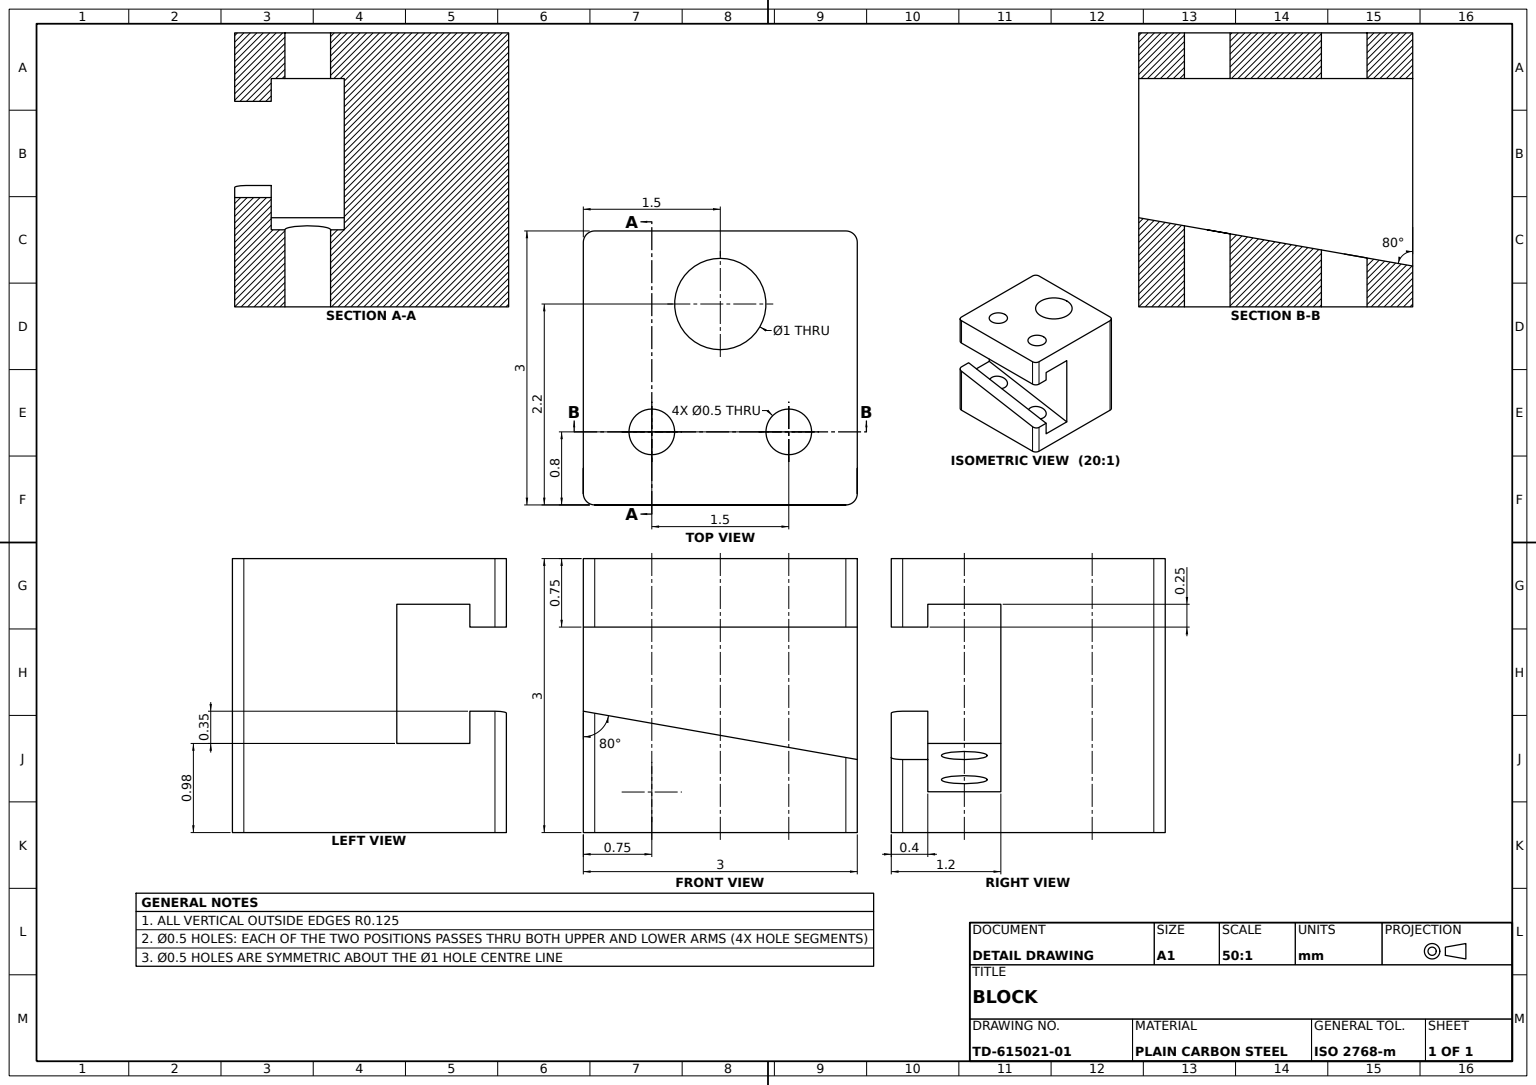
from build123d import *

# Parameters (mm, degrees)
C_PROFILE_SKETCH_W         = 3
C_PROFILE_SKETCH_H         = 3
C_BODY_EXTRUDE_3MM_DEPTH   = 1.5
ANGLED_JAW_CUT_10DEG_DEPTH = 1.2
JAW_NOTCH_CUT_DEPTH        = 0.8
EDGE_FILLETS_R0_125_R      = 0.125
MOUNTING_HOLES_SKETCH_R    = 0.5
MOUNTING_HOLES_SKETCH_R_2  = 0.25
MOUNTING_HOLES_3X_DEPTH    = 4.674234614


with BuildPart() as part:
    # C-Profile Sketch → C-Body Extrude 3mm (new, symmetric)
    with BuildSketch(Plane.XY):
        Rectangle(C_PROFILE_SKETCH_W, C_PROFILE_SKETCH_H)
    extrude(amount=C_BODY_EXTRUDE_3MM_DEPTH, both=True)

    # Angled Jaw Sketch → Angled Jaw Cut 10deg (cut)
    with BuildSketch(Plane.XY.offset(1.5)):
        Polygon((1.5, -0.7), (-1.5, -0.171019058), (-1.5, 0.75), (1.5, 0.75), align=None)
    extrude(amount=-ANGLED_JAW_CUT_10DEG_DEPTH, mode=Mode.SUBTRACT)

    # Jaw Notch Sketch → Jaw Notch Cut (cut)
    with BuildSketch(Plane.XY.offset(0.3)):
        Polygon((1.5, -0.7), (1.5, -1.053), (-1.5, -0.524019058), (-1.5, 1), (1.5, 1), align=None)
    extrude(amount=JAW_NOTCH_CUT_DEPTH, mode=Mode.SUBTRACT)

    # Edge Fillets R0.125
    edge_fillets_r0_125_edges = [part.edges().sort_by_distance(p)[0] for p in [
        (-1.5, 1.125, 1.5),
        (-1.5, -0.835509529, 1.5),
        (1.5, 1.125, 1.5),
        (1.5, -1.1, 1.5),
        (-1.5, 0, -1.5),
        (1.5, 0, -1.5),
    ]]
    fillet(edge_fillets_r0_125_edges, radius=EDGE_FILLETS_R0_125_R)

    # Mounting Holes Sketch → Mounting Holes 3x (cut, through all)
    with BuildSketch(Plane(origin=(0, 1.5, 0), x_dir=(1, 0, 0), z_dir=(0, 1, 0))):
        with Locations(Location((0, 0.7, 0), (0, 0, 270))):
            Circle(MOUNTING_HOLES_SKETCH_R)
        with Locations(Location((0.75, -0.7, 0), (0, 0, 270))):
            Circle(MOUNTING_HOLES_SKETCH_R_2)
        with Locations(Location((-0.75, -0.7, 0), (0, 0, 270))):
            Circle(MOUNTING_HOLES_SKETCH_R_2)
    extrude(amount=-MOUNTING_HOLES_3X_DEPTH, mode=Mode.SUBTRACT)


solid = part.part
